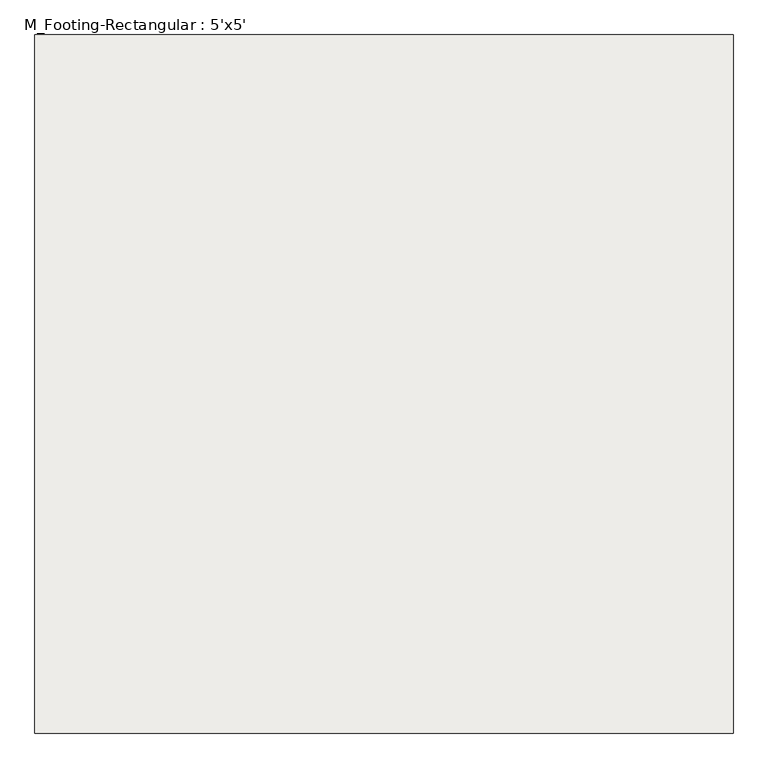
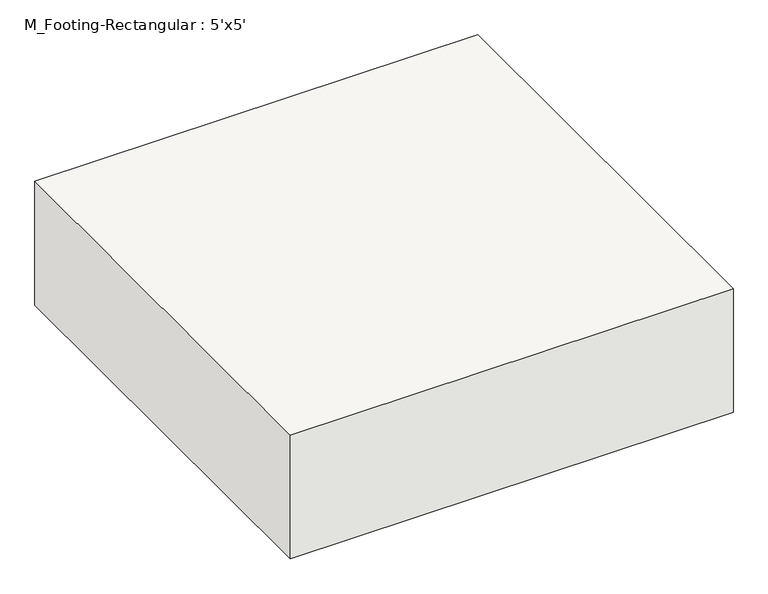
"""IFC4 building model written with IfcOpenShell, lengths in millimetres: slab geometry, M_Footing-Rectangular : 5'x5'."""

from ifc_helpers import new_model, si_unit, frame, origin, place, context, project, spatial, polyline, outline, extrude, source, transform, mapped, element, save


def m_footing_rectangular_5_x5_4154a230(model_context):
    return source(origin(), model_context, "Body", "SweptSolid", [
        extrude(outline(polyline([(762.0, 762.0), (762.0, -762.0), (-762.0, -762.0), (-762.0, 762.0), (762.0, 762.0)])), frame((0.0, 0.0, -450.0), z_axis=(0.0, 0.0, 1.0), x_axis=(1.0, 0.0, 0.0)), (0.0, 0.0, 1.0), 450.0),
    ])


if __name__ == "__main__":
    model = new_model("IFC4")
    model_context = context("Model", 3, world=origin())
    ifc_project = project(units=[si_unit("LENGTHUNIT", "METRE", prefix="MILLI")], contexts=[model_context])
    site = spatial("IfcSite", under=ifc_project)
    building = spatial("IfcBuilding", under=site)
    placement = place(None, origin())
    m_footing_rectangular_5_x5_shape = m_footing_rectangular_5_x5_4154a230(model_context)
    element("IfcSlab", 1, ObjectType="M_Footing-Rectangular : 5'x5'", at=placement, inside=building, context=model_context, shape_type="MappedRepresentation", body=[
        mapped(m_footing_rectangular_5_x5_shape, transform((0.0, 0.0, 0.0), x_axis=(1.0, 0.0, 0.0), y_axis=(0.0, 1.0, 0.0), z_axis=(0.0, 0.0, 1.0))),
    ])
    save(model, "model.ifc")

# Revit data of these elements
# Type "M_Footing-Rectangular : 5'x5'"
#   Width = 5' - 0"
#   Length = 5' - 0"
#   Foundation Thickness = 1' - 5.71654"
#   Structural Material [instance default] = Concrete, Cast-in-Place gray
#   Assembly Code = ""
# Element 1 (IfcSlab, "M_Footing-Rectangular : 5'x5'")
#   Materials on its faces: "Concrete, Cast-in-Place gray"
# Materials
#   "Concrete, Cast-in-Place gray": class "Concrete", colour RGB 192 192 192, transparency 0, Description = "Cast-in-place concrete", Cost = 0
